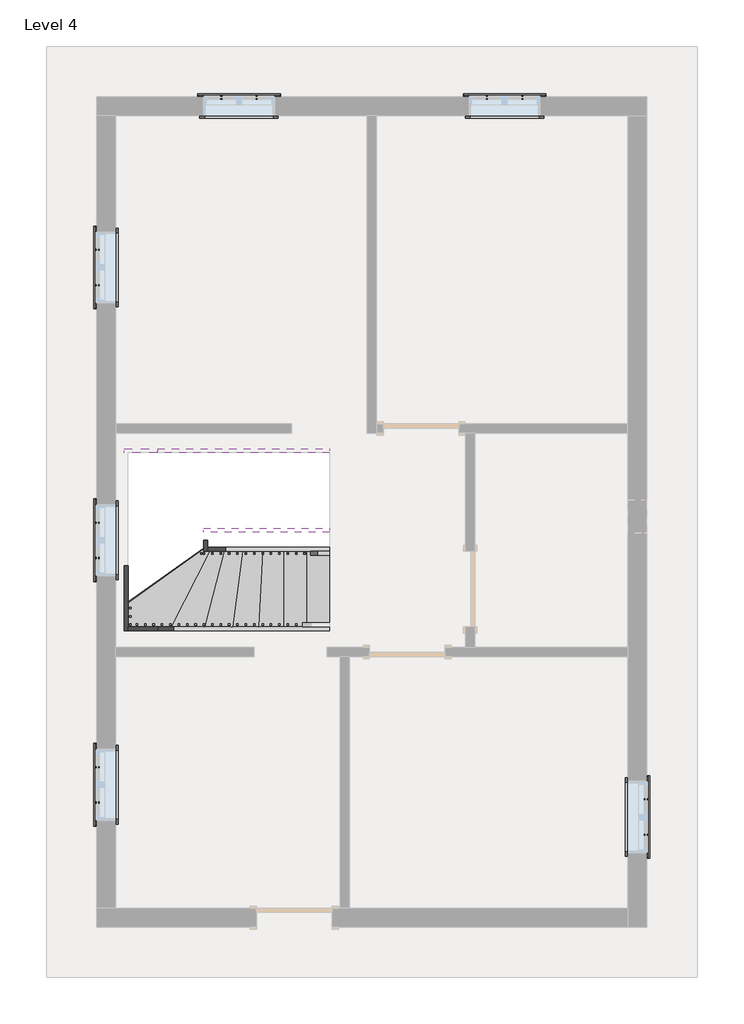
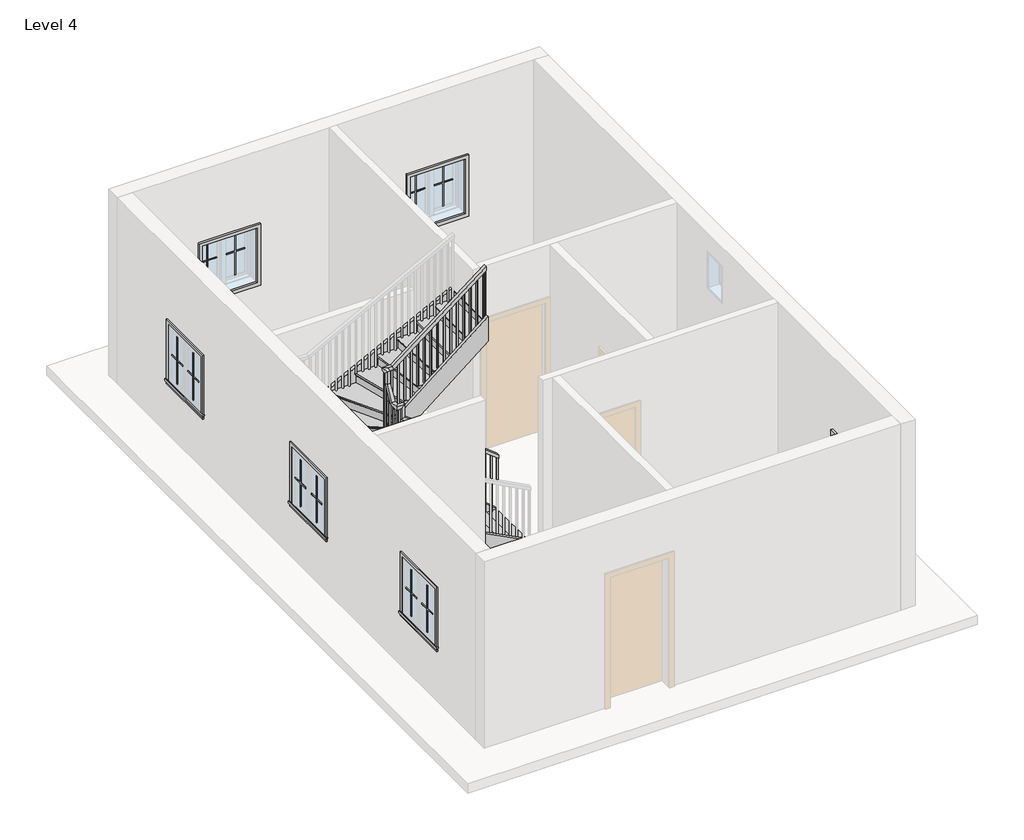
# One storey, part 2 of 2: 24 proxies, 8 members, 1 railing, 1 stair flight.
"""IFC4 building model written with IfcOpenShell, lengths in millimetres."""

from ifc_helpers import new_model, si_unit, frame, origin, place, context, project, spatial, polyline, outline, extrude, faceted_brep, transform, mapped, element, save
from components import muntin_pattern_2x2_muntin_pattern_2x2_b3fe6957, muntin_pattern_2x2_muntin_pattern_2x2_3e0ecaf2, trim_window_exterior_flat_with_sill_41619996, trim_window_interior_flat_picture_frame_51c85655, stair_flight_c61886c8

model = new_model("IFC4")

# Units and contexts
model_context = context("Model", 3, world=origin())
ifc_project = project(units=[si_unit("LENGTHUNIT", "METRE", prefix="MILLI")], contexts=[model_context])

# Site, building, storey
site = spatial("IfcSite", under=ifc_project)
building = spatial("IfcBuilding", under=site)
storey = spatial("IfcBuildingStorey", under=building, Name="Level 4", Elevation=6400.8)

# Proxies
placement = place(None, origin())
muntin_pattern_2x2_muntin_pattern_2x2_shape = muntin_pattern_2x2_muntin_pattern_2x2_b3fe6957(model_context)
element("IfcBuildingElementProxy", 1, Name="Muntin Pattern_2x2 : Muntin Pattern_2x2", ObjectType="Muntin Pattern_2x2 : Muntin Pattern_2x2", at=placement, inside=storey, context=model_context, shape_type="MappedRepresentation", body=[
    mapped(muntin_pattern_2x2_muntin_pattern_2x2_shape, transform((-3096.8324167, 5150.2179147, 7385.05), x_axis=(1.0, 0.0, 0.0), y_axis=(0.0, 1.0, 0.0), z_axis=(0.0, 0.0, 1.0))),
])
element("IfcBuildingElementProxy", 2, Name="Muntin Pattern_2x2 : Muntin Pattern_2x2", ObjectType="Muntin Pattern_2x2 : Muntin Pattern_2x2", at=placement, inside=storey, context=model_context, shape_type="MappedRepresentation", body=[
    mapped(muntin_pattern_2x2_muntin_pattern_2x2_shape, transform((122.6175833, 5150.2179147, 7385.05), x_axis=(1.0, 0.0, 0.0), y_axis=(0.0, 1.0, 0.0), z_axis=(0.0, 0.0, 1.0))),
])
element("IfcBuildingElementProxy", 3, Name="Muntin Pattern_2x2 : Muntin Pattern_2x2", ObjectType="Muntin Pattern_2x2 : Muntin Pattern_2x2", at=placement, inside=storey, context=model_context, shape_type="MappedRepresentation", body=[
    mapped(muntin_pattern_2x2_muntin_pattern_2x2_shape, transform((2051.4300833, -3350.8445853, 7385.05), x_axis=(0.0, -1.0, 0.0), y_axis=(1.0, 0.0, 0.0), z_axis=(0.0, 0.0, 1.0))),
])
element("IfcBuildingElementProxy", 4, Name="Muntin Pattern_2x2 : Muntin Pattern_2x2", ObjectType="Muntin Pattern_2x2 : Muntin Pattern_2x2", at=placement, inside=storey, context=model_context, shape_type="MappedRepresentation", body=[
    mapped(muntin_pattern_2x2_muntin_pattern_2x2_shape, transform((-4597.0199167, -426.6695853, 7385.05), x_axis=(0.0, 1.0, 0.0), y_axis=(-1.0, 0.0, 0.0), z_axis=(0.0, 0.0, 1.0))),
])
element("IfcBuildingElementProxy", 5, Name="Muntin Pattern_2x2 : Muntin Pattern_2x2", ObjectType="Muntin Pattern_2x2 : Muntin Pattern_2x2", at=placement, inside=storey, context=model_context, shape_type="MappedRepresentation", body=[
    mapped(muntin_pattern_2x2_muntin_pattern_2x2_shape, transform((-4597.0199167, -3388.9445853, 7385.05), x_axis=(0.0, 1.0, 0.0), y_axis=(-1.0, 0.0, 0.0), z_axis=(0.0, 0.0, 1.0))),
])
element("IfcBuildingElementProxy", 6, Name="Muntin Pattern_2x2 : Muntin Pattern_2x2", ObjectType="Muntin Pattern_2x2 : Muntin Pattern_2x2", at=placement, inside=storey, context=model_context, shape_type="MappedRepresentation", body=[
    mapped(muntin_pattern_2x2_muntin_pattern_2x2_shape, transform((-4597.0199167, 2878.5054147, 7385.05), x_axis=(0.0, 1.0, 0.0), y_axis=(-1.0, 0.0, 0.0), z_axis=(0.0, 0.0, 1.0))),
])
muntin_pattern_2x2_muntin_pattern_2x2_2_shape = muntin_pattern_2x2_muntin_pattern_2x2_3e0ecaf2(model_context)
element("IfcBuildingElementProxy", 7, Name="Muntin Pattern_2x2 : Muntin Pattern_2x2", ObjectType="Muntin Pattern_2x2 : Muntin Pattern_2x2", at=placement, inside=storey, context=model_context, shape_type="MappedRepresentation", body=[
    mapped(muntin_pattern_2x2_muntin_pattern_2x2_2_shape, transform((-2668.2074167, 5150.2179147, 7385.05), x_axis=(-1.0, 0.0, 0.0), y_axis=(0.0, -1.0, 0.0), z_axis=(0.0, 0.0, 1.0))),
])
element("IfcBuildingElementProxy", 8, Name="Muntin Pattern_2x2 : Muntin Pattern_2x2", ObjectType="Muntin Pattern_2x2 : Muntin Pattern_2x2", at=placement, inside=storey, context=model_context, shape_type="MappedRepresentation", body=[
    mapped(muntin_pattern_2x2_muntin_pattern_2x2_2_shape, transform((551.2425833, 5150.2179147, 7385.05), x_axis=(-1.0, 0.0, 0.0), y_axis=(0.0, -1.0, 0.0), z_axis=(0.0, 0.0, 1.0))),
])
element("IfcBuildingElementProxy", 9, Name="Muntin Pattern_2x2 : Muntin Pattern_2x2", ObjectType="Muntin Pattern_2x2 : Muntin Pattern_2x2", at=placement, inside=storey, context=model_context, shape_type="MappedRepresentation", body=[
    mapped(muntin_pattern_2x2_muntin_pattern_2x2_2_shape, transform((2051.4300833, -3779.4695853, 7385.05), x_axis=(0.0, 1.0, 0.0), y_axis=(-1.0, 0.0, 0.0), z_axis=(0.0, 0.0, 1.0))),
])
element("IfcBuildingElementProxy", 10, Name="Muntin Pattern_2x2 : Muntin Pattern_2x2", ObjectType="Muntin Pattern_2x2 : Muntin Pattern_2x2", at=placement, inside=storey, context=model_context, shape_type="MappedRepresentation", body=[
    mapped(muntin_pattern_2x2_muntin_pattern_2x2_2_shape, transform((-4597.0199167, 1.9554147, 7385.05), x_axis=(0.0, -1.0, 0.0), y_axis=(1.0, 0.0, 0.0), z_axis=(0.0, 0.0, 1.0))),
])
element("IfcBuildingElementProxy", 11, Name="Muntin Pattern_2x2 : Muntin Pattern_2x2", ObjectType="Muntin Pattern_2x2 : Muntin Pattern_2x2", at=placement, inside=storey, context=model_context, shape_type="MappedRepresentation", body=[
    mapped(muntin_pattern_2x2_muntin_pattern_2x2_2_shape, transform((-4597.0199167, -2960.3195853, 7385.05), x_axis=(0.0, -1.0, 0.0), y_axis=(1.0, 0.0, 0.0), z_axis=(0.0, 0.0, 1.0))),
])
element("IfcBuildingElementProxy", 12, Name="Muntin Pattern_2x2 : Muntin Pattern_2x2", ObjectType="Muntin Pattern_2x2 : Muntin Pattern_2x2", at=placement, inside=storey, context=model_context, shape_type="MappedRepresentation", body=[
    mapped(muntin_pattern_2x2_muntin_pattern_2x2_2_shape, transform((-4597.0199167, 3307.1304147, 7385.05), x_axis=(0.0, -1.0, 0.0), y_axis=(1.0, 0.0, 0.0), z_axis=(0.0, 0.0, 1.0))),
])
trim_window_exterior_flat_with_sill_shape = trim_window_exterior_flat_with_sill_41619996(model_context)
element("IfcBuildingElementProxy", 13, Name="Trim-Window-Exterior-Flat : with Sill", ObjectType="Trim-Window-Exterior-Flat : with Sill", at=placement, inside=storey, context=model_context, shape_type="MappedRepresentation", body=[
    mapped(trim_window_exterior_flat_with_sill_shape, transform((-2882.5199167, 5159.7429147, 8229.6), x_axis=(-1.0, 0.0, 0.0), y_axis=(0.0, 0.0, 1.0), z_axis=(0.0, 1.0, 0.0))),
])
element("IfcBuildingElementProxy", 14, Name="Trim-Window-Exterior-Flat : with Sill", ObjectType="Trim-Window-Exterior-Flat : with Sill", at=placement, inside=storey, context=model_context, shape_type="MappedRepresentation", body=[
    mapped(trim_window_exterior_flat_with_sill_shape, transform((336.9300833, 5159.7429147, 8229.6), x_axis=(-1.0, 0.0, 0.0), y_axis=(0.0, 0.0, 1.0), z_axis=(0.0, 1.0, 0.0))),
])
element("IfcBuildingElementProxy", 15, Name="Trim-Window-Exterior-Flat : with Sill", ObjectType="Trim-Window-Exterior-Flat : with Sill", at=placement, inside=storey, context=model_context, shape_type="MappedRepresentation", body=[
    mapped(trim_window_exterior_flat_with_sill_shape, transform((2060.9550833, -3565.1570853, 8229.6), x_axis=(0.0, 1.0, 0.0), y_axis=(0.0, 0.0, 1.0), z_axis=(1.0, 0.0, 0.0))),
])
element("IfcBuildingElementProxy", 16, Name="Trim-Window-Exterior-Flat : with Sill", ObjectType="Trim-Window-Exterior-Flat : with Sill", at=placement, inside=storey, context=model_context, shape_type="MappedRepresentation", body=[
    mapped(trim_window_exterior_flat_with_sill_shape, transform((-4606.5449167, -212.3570853, 8229.6), x_axis=(0.0, -1.0, 0.0), y_axis=(0.0, 0.0, 1.0), z_axis=(-1.0, 0.0, 0.0))),
])
element("IfcBuildingElementProxy", 17, Name="Trim-Window-Exterior-Flat : with Sill", ObjectType="Trim-Window-Exterior-Flat : with Sill", at=placement, inside=storey, context=model_context, shape_type="MappedRepresentation", body=[
    mapped(trim_window_exterior_flat_with_sill_shape, transform((-4606.5449167, -3174.6320853, 8229.6), x_axis=(0.0, -1.0, 0.0), y_axis=(0.0, 0.0, 1.0), z_axis=(-1.0, 0.0, 0.0))),
])
element("IfcBuildingElementProxy", 18, Name="Trim-Window-Exterior-Flat : with Sill", ObjectType="Trim-Window-Exterior-Flat : with Sill", at=placement, inside=storey, context=model_context, shape_type="MappedRepresentation", body=[
    mapped(trim_window_exterior_flat_with_sill_shape, transform((-4606.5449167, 3092.8179147, 8229.6), x_axis=(0.0, -1.0, 0.0), y_axis=(0.0, 0.0, 1.0), z_axis=(-1.0, 0.0, 0.0))),
])
trim_window_interior_flat_picture_frame_shape = trim_window_interior_flat_picture_frame_51c85655(model_context)
element("IfcBuildingElementProxy", 19, Name="Trim-Window-Interior-Flat : Picture Frame", ObjectType="Trim-Window-Interior-Flat : Picture Frame", at=placement, inside=storey, context=model_context, shape_type="MappedRepresentation", body=[
    mapped(trim_window_interior_flat_picture_frame_shape, transform((-2882.5199167, 4931.1429147, 8229.6), x_axis=(1.0, 0.0, 0.0), y_axis=(0.0, 0.0, 1.0), z_axis=(0.0, -1.0, 0.0))),
])
element("IfcBuildingElementProxy", 20, Name="Trim-Window-Interior-Flat : Picture Frame", ObjectType="Trim-Window-Interior-Flat : Picture Frame", at=placement, inside=storey, context=model_context, shape_type="MappedRepresentation", body=[
    mapped(trim_window_interior_flat_picture_frame_shape, transform((336.9300833, 4931.1429147, 8229.6), x_axis=(1.0, 0.0, 0.0), y_axis=(0.0, 0.0, 1.0), z_axis=(0.0, -1.0, 0.0))),
])
element("IfcBuildingElementProxy", 21, Name="Trim-Window-Interior-Flat : Picture Frame", ObjectType="Trim-Window-Interior-Flat : Picture Frame", at=placement, inside=storey, context=model_context, shape_type="MappedRepresentation", body=[
    mapped(trim_window_interior_flat_picture_frame_shape, transform((1832.3550833, -3565.1570853, 8229.6), x_axis=(0.0, -1.0, 0.0), y_axis=(0.0, 0.0, 1.0), z_axis=(-1.0, 0.0, 0.0))),
])
element("IfcBuildingElementProxy", 22, Name="Trim-Window-Interior-Flat : Picture Frame", ObjectType="Trim-Window-Interior-Flat : Picture Frame", at=placement, inside=storey, context=model_context, shape_type="MappedRepresentation", body=[
    mapped(trim_window_interior_flat_picture_frame_shape, transform((-4377.9449167, -212.3570853, 8229.6), x_axis=(0.0, 1.0, 0.0), y_axis=(0.0, 0.0, 1.0), z_axis=(1.0, 0.0, 0.0))),
])
element("IfcBuildingElementProxy", 23, Name="Trim-Window-Interior-Flat : Picture Frame", ObjectType="Trim-Window-Interior-Flat : Picture Frame", at=placement, inside=storey, context=model_context, shape_type="MappedRepresentation", body=[
    mapped(trim_window_interior_flat_picture_frame_shape, transform((-4377.9449167, -3174.6320853, 8229.6), x_axis=(0.0, 1.0, 0.0), y_axis=(0.0, 0.0, 1.0), z_axis=(1.0, 0.0, 0.0))),
])
element("IfcBuildingElementProxy", 24, Name="Trim-Window-Interior-Flat : Picture Frame", ObjectType="Trim-Window-Interior-Flat : Picture Frame", at=placement, inside=storey, context=model_context, shape_type="MappedRepresentation", body=[
    mapped(trim_window_interior_flat_picture_frame_shape, transform((-4377.9449167, 3092.8179147, 8229.6), x_axis=(0.0, 1.0, 0.0), y_axis=(0.0, 0.0, 1.0), z_axis=(1.0, 0.0, 0.0))),
])

# Members
element("IfcMember", 25, ObjectType="Stringer - 2\" Width", at=placement, inside=storey, context=model_context, shape_type="SweptSolid", body=[
    extrude(outline(polyline([(6400.8, -1783.4132248), (6630.439954, -1783.4132248), (7706.1956453, -3870.8304165), (7363.300629, -3870.8304165), (6400.8, -2003.1755424), (6400.8, -1783.4132248)])), frame((0.0, -1310.9070853, 0.0), z_axis=(0.0, 1.0, 0.0), x_axis=(0.0, 0.0, 1.0)), (0.0, 0.0, 1.0), 50.8),
])
element("IfcMember", 26, ObjectType="Stringer - 2\" Width", at=placement, inside=storey, context=model_context, shape_type="SweptSolid", body=[
    extrude(outline(polyline([(-3870.8304165, -1260.1070853), (-3870.8304165, -1310.9070853), (-4225.5449167, -1310.9070853), (-4225.5449167, -1260.1070853), (-3870.8304165, -1260.1070853)])), frame((0.0, 0.0, 7363.300629), z_axis=(0.0, 0.0, 1.0), x_axis=(1.0, 0.0, 0.0)), (0.0, 0.0, 1.0), 342.8950162),
])
element("IfcMember", 27, ObjectType="Stringer - 2\" Width", at=placement, inside=storey, context=model_context, shape_type="SweptSolid", body=[
    extrude(outline(polyline([(-1310.9070853, 7401.3956453), (-1310.9070853, 7689.8952212), (811.1127974, 8370.7972697), (848.0929147, 8370.7972697), (848.0929147, 8039.7682298), (-1141.3846024, 7401.3956453), (-1310.9070853, 7401.3956453)])), frame((-4276.3449167, 0.0, 0.0), z_axis=(1.0, 0.0, 0.0), x_axis=(0.0, 1.0, 0.0)), (0.0, 0.0, 1.0), 50.8),
])
element("IfcMember", 28, ObjectType="Stringer - 2\" Width", at=placement, inside=storey, context=model_context, shape_type="SweptSolid", body=[
    extrude(outline(polyline([(-4276.3449167, 848.0929147), (-4276.3449167, 898.8929147), (-3870.8304165, 898.8929147), (-3870.8304165, 848.0929147), (-4276.3449167, 848.0929147)])), frame((0.0, 0.0, 8050.6904473), z_axis=(0.0, 0.0, 1.0), x_axis=(1.0, 0.0, 0.0)), (0.0, 0.0, 1.0), 320.1068224),
])
element("IfcMember", 29, ObjectType="Stringer - 2\" Width", at=placement, inside=storey, context=model_context, shape_type="SweptSolid", body=[
    extrude(outline(polyline([(8370.7972697, -3870.8304165), (8050.6904473, -3870.8304165), (9126.4461385, -1783.4132248), (9446.5529609, -1783.4132248), (8370.7972697, -3870.8304165)])), frame((0.0, 848.0929147, 0.0), z_axis=(0.0, 1.0, 0.0), x_axis=(0.0, 0.0, 1.0)), (0.0, 0.0, 1.0), 50.8),
])
element("IfcMember", 30, ObjectType="Stringer - 2\" Width", at=placement, inside=storey, context=model_context, shape_type="SweptSolid", body=[
    extrude(outline(polyline([(6400.8, -1783.4132248), (6576.9764461, -1783.4132248), (7781.218648, -3260.3449167), (7387.9410923, -3260.3449167), (6400.8, -2049.6748694), (6400.8, -1783.4132248)])), frame((0.0, -345.7070853, 0.0), z_axis=(0.0, 1.0, 0.0), x_axis=(0.0, 0.0, 1.0)), (0.0, 0.0, 1.0), 50.8),
])
element("IfcMember", 31, ObjectType="Stringer - 2\" Width", at=placement, inside=storey, context=model_context, shape_type="SweptSolid", body=[
    extrude(outline(polyline([(-345.7070853, 7429.3617647), (-345.7070853, 7974.0682978), (-139.0699679, 8326.9409689), (-117.1070853, 8326.9409689), (-117.1070853, 7761.265107), (-311.464868, 7429.3617647), (-345.7070853, 7429.3617647)])), frame((-3311.1449167, 0.0, 0.0), z_axis=(1.0, 0.0, 0.0), x_axis=(0.0, 1.0, 0.0)), (0.0, 0.0, 1.0), 50.8),
])
element("IfcMember", 32, ObjectType="Stringer - 2\" Width", at=placement, inside=storey, context=model_context, shape_type="SweptSolid", body=[
    extrude(outline(polyline([(8326.9409689, -3311.1449167), (7933.6634131, -3311.1449167), (9179.3262875, -1783.4132248), (9572.6038432, -1783.4132248), (8326.9409689, -3311.1449167)])), frame((0.0, -117.1070853, 0.0), z_axis=(0.0, 1.0, 0.0), x_axis=(0.0, 0.0, 1.0)), (0.0, 0.0, 1.0), 50.8),
])

# Railing
element("IfcRailing", 33, ObjectType="Handrail - Rectangular", at=placement, inside=storey, context=model_context, shape_type="SolidModel", body=[
    faceted_brep([(-1783.4132248, -396.5070853, 7484.5333333), (-1783.4132248, -396.5070853, 7420.2000346), (-1783.4132248, -345.7070853, 7420.2000346), (-1783.4132248, -345.7070853, 7484.5333333), (-3234.9449167, -396.5070853, 8612.4191036), (-3285.7449167, -396.5070853, 8587.5590024), (-3285.7449167, -345.7070853, 8587.5590024), (-3234.9449167, -345.7070853, 8612.4191036), (-3234.9449167, -396.5070853, 8815.4281882), (-3285.7449167, -396.5070853, 8764.6281882), (-3285.7449167, -345.7070853, 8764.6281882), (-3234.9449167, -345.7070853, 8815.4281882), (-3361.9449167, -396.5070853, 8815.4281882), (-3361.9449167, -396.5070853, 8764.6281882), (-3311.1449167, -345.7070853, 8764.6281882), (-3311.1449167, -345.7070853, 8815.4281882), (-3361.9449167, -269.5070853, 8815.4281882), (-3361.9449167, -240.3857515, 8764.6281882), (-3311.1449167, -240.3857515, 8764.6281882), (-3311.1449167, -269.5070853, 8815.4281882), (-3361.9449167, -142.5070853, 9032.3051451), (-3361.9449167, -91.7070853, 9018.5256424), (-3311.1449167, -91.7070853, 9018.5256424), (-3311.1449167, -142.5070853, 9032.3051451), (-3361.9449167, -142.5070853, 9235.3142297), (-3361.9449167, -91.7070853, 9184.5142297), (-3311.1449167, -91.7070853, 9184.5142297), (-3311.1449167, -142.5070853, 9235.3142297), (-3361.9449167, -15.5070853, 9235.3142297), (-3361.9449167, -15.5070853, 9184.5142297), (-3311.1449167, -66.3070853, 9184.5142297), (-3311.1449167, -66.3070853, 9235.3142297), (-3234.9449167, -15.5070853, 9235.3142297), (-3217.5282487, -15.5070853, 9184.5142297), (-3217.5282487, -66.3070853, 9184.5142297), (-3234.9449167, -66.3070853, 9235.3142297), (-1783.4132248, -15.5070853, 10363.2), (-1783.4132248, -66.3070853, 10363.2), (-1783.4132248, -66.3070853, 10298.8667013), (-1783.4132248, -15.5070853, 10298.8667013)], [[[0, 1, 2, 3]], [[1, 0, 4, 5]], [[2, 1, 5, 6]], [[3, 2, 6, 7]], [[0, 3, 7, 4]], [[5, 4, 8, 9]], [[6, 5, 9, 10]], [[7, 6, 10, 11]], [[4, 7, 11, 8]], [[9, 8, 12, 13]], [[10, 9, 13, 14]], [[11, 10, 14, 15]], [[8, 11, 15, 12]], [[13, 12, 16, 17]], [[14, 13, 17, 18]], [[15, 14, 18, 19]], [[12, 15, 19, 16]], [[17, 16, 20, 21]], [[18, 17, 21, 22]], [[19, 18, 22, 23]], [[16, 19, 23, 20]], [[21, 20, 24, 25]], [[22, 21, 25, 26]], [[23, 22, 26, 27]], [[20, 23, 27, 24]], [[25, 24, 28, 29]], [[26, 25, 29, 30]], [[27, 26, 30, 31]], [[24, 27, 31, 28]], [[29, 28, 32, 33]], [[30, 29, 33, 34]], [[31, 30, 34, 35]], [[28, 31, 35, 32]], [[36, 37, 38, 39]], [[33, 32, 36, 39]], [[34, 33, 39, 38]], [[35, 34, 38, 37]], [[32, 35, 37, 36]]]),
    extrude(outline(polyline([(10283.6316852, -1803.0199167), (10268.8292361, -1822.0699167), (9279.4666667, -1822.0699167), (9279.4666667, -1803.0199167), (10283.6316852, -1803.0199167)])), frame((0.0, -50.4320853, 0.0), z_axis=(0.0, 1.0, 0.0), x_axis=(0.0, 0.0, 1.0)), (0.0, 0.0, 1.0), 19.05),
    extrude(outline(polyline([(10204.6852902, -1904.6199167), (10189.8828411, -1923.6699167), (9279.4666667, -1923.6699167), (9279.4666667, -1904.6199167), (10204.6852902, -1904.6199167)])), frame((0.0, -50.4320853, 0.0), z_axis=(0.0, 1.0, 0.0), x_axis=(0.0, 0.0, 1.0)), (0.0, 0.0, 1.0), 19.05),
    extrude(outline(polyline([(10125.7388952, -2006.2199167), (10110.9364462, -2025.2699167), (9279.4666667, -2025.2699167), (9279.4666667, -2006.2199167), (10125.7388952, -2006.2199167)])), frame((0.0, -50.4320853, 0.0), z_axis=(0.0, 1.0, 0.0), x_axis=(0.0, 0.0, 1.0)), (0.0, 0.0, 1.0), 19.05),
    extrude(outline(polyline([(10046.7925003, -2107.8199167), (10031.9900512, -2126.8699167), (9110.1333333, -2126.8699167), (9110.1333333, -2107.8199167), (10046.7925003, -2107.8199167)])), frame((0.0, -50.4320853, 0.0), z_axis=(0.0, 1.0, 0.0), x_axis=(0.0, 0.0, 1.0)), (0.0, 0.0, 1.0), 19.05),
    extrude(outline(polyline([(9967.8461053, -2209.4199167), (9953.0436562, -2228.4699167), (9110.1333333, -2228.4699167), (9110.1333333, -2209.4199167), (9967.8461053, -2209.4199167)])), frame((0.0, -50.4320853, 0.0), z_axis=(0.0, 1.0, 0.0), x_axis=(0.0, 0.0, 1.0)), (0.0, 0.0, 1.0), 19.05),
    extrude(outline(polyline([(9888.8997103, -2311.0199167), (9874.0972613, -2330.0699167), (9110.1333333, -2330.0699167), (9110.1333333, -2311.0199167), (9888.8997103, -2311.0199167)])), frame((0.0, -50.4320853, 0.0), z_axis=(0.0, 1.0, 0.0), x_axis=(0.0, 0.0, 1.0)), (0.0, 0.0, 1.0), 19.05),
    extrude(outline(polyline([(9809.9533154, -2412.6199167), (9795.1508663, -2431.6699167), (8940.8, -2431.6699167), (8940.8, -2412.6199167), (9809.9533154, -2412.6199167)])), frame((0.0, -50.4320853, 0.0), z_axis=(0.0, 1.0, 0.0), x_axis=(0.0, 0.0, 1.0)), (0.0, 0.0, 1.0), 19.05),
    extrude(outline(polyline([(9731.0069204, -2514.2199167), (9716.2044713, -2533.2699167), (8940.8, -2533.2699167), (8940.8, -2514.2199167), (9731.0069204, -2514.2199167)])), frame((0.0, -50.4320853, 0.0), z_axis=(0.0, 1.0, 0.0), x_axis=(0.0, 0.0, 1.0)), (0.0, 0.0, 1.0), 19.05),
    extrude(outline(polyline([(9652.0605254, -2615.8199167), (9637.2580764, -2634.8699167), (8771.4666667, -2634.8699167), (8771.4666667, -2615.8199167), (9652.0605254, -2615.8199167)])), frame((0.0, -50.4320853, 0.0), z_axis=(0.0, 1.0, 0.0), x_axis=(0.0, 0.0, 1.0)), (0.0, 0.0, 1.0), 19.05),
    extrude(outline(polyline([(9573.1141304, -2717.4199167), (9558.3116814, -2736.4699167), (8771.4666667, -2736.4699167), (8771.4666667, -2717.4199167), (9573.1141304, -2717.4199167)])), frame((0.0, -50.4320853, 0.0), z_axis=(0.0, 1.0, 0.0), x_axis=(0.0, 0.0, 1.0)), (0.0, 0.0, 1.0), 19.05),
    extrude(outline(polyline([(9494.1677355, -2819.0199167), (9479.3652864, -2838.0699167), (8771.4666667, -2838.0699167), (8771.4666667, -2819.0199167), (9494.1677355, -2819.0199167)])), frame((0.0, -50.4320853, 0.0), z_axis=(0.0, 1.0, 0.0), x_axis=(0.0, 0.0, 1.0)), (0.0, 0.0, 1.0), 19.05),
    extrude(outline(polyline([(9415.2213405, -2920.6199167), (9400.4188914, -2939.6699167), (8602.1333333, -2939.6699167), (8602.1333333, -2920.6199167), (9415.2213405, -2920.6199167)])), frame((0.0, -50.4320853, 0.0), z_axis=(0.0, 1.0, 0.0), x_axis=(0.0, 0.0, 1.0)), (0.0, 0.0, 1.0), 19.05),
    extrude(outline(polyline([(9336.2749455, -3022.2199167), (9321.4724965, -3041.2699167), (8602.1333333, -3041.2699167), (8602.1333333, -3022.2199167), (9336.2749455, -3022.2199167)])), frame((0.0, -50.4320853, 0.0), z_axis=(0.0, 1.0, 0.0), x_axis=(0.0, 0.0, 1.0)), (0.0, 0.0, 1.0), 19.05),
    extrude(outline(polyline([(9257.3285506, -3123.8199167), (9242.5261015, -3142.8699167), (8432.8, -3142.8699167), (8432.8, -3123.8199167), (9257.3285506, -3123.8199167)])), frame((0.0, -50.4320853, 0.0), z_axis=(0.0, 1.0, 0.0), x_axis=(0.0, 0.0, 1.0)), (0.0, 0.0, 1.0), 19.05),
    extrude(outline(polyline([(9178.3821556, -3225.4199167), (9163.5797065, -3244.4699167), (8432.8, -3244.4699167), (8432.8, -3225.4199167), (9178.3821556, -3225.4199167)])), frame((0.0, -50.4320853, 0.0), z_axis=(0.0, 1.0, 0.0), x_axis=(0.0, 0.0, 1.0)), (0.0, 0.0, 1.0), 19.05),
    extrude(outline(polyline([(-3327.0199167, -75.8320853), (-3346.0699167, -75.8320853), (-3346.0699167, -56.7820853), (-3327.0199167, -56.7820853), (-3327.0199167, -75.8320853)])), frame((0.0, 0.0, 8094.1333333), z_axis=(0.0, 0.0, 1.0), x_axis=(1.0, 0.0, 0.0)), (0.0, 0.0, 1.0), 1090.3808964),
    extrude(outline(polyline([(-177.4320853, 8872.1336964), (-158.3820853, 8904.66524), (-158.3820853, 7924.8), (-177.4320853, 7924.8), (-177.4320853, 8872.1336964)])), frame((-3346.0699167, 0.0, 0.0), z_axis=(1.0, 0.0, 0.0), x_axis=(0.0, 1.0, 0.0)), (0.0, 0.0, 1.0), 19.05),
    extrude(outline(polyline([(-279.0320853, 8698.6321309), (-259.9820853, 8731.1636744), (-259.9820853, 7755.4666667), (-279.0320853, 7755.4666667), (-279.0320853, 8698.6321309)])), frame((-3346.0699167, 0.0, 0.0), z_axis=(1.0, 0.0, 0.0), x_axis=(0.0, 1.0, 0.0)), (0.0, 0.0, 1.0), 19.05),
    extrude(outline(polyline([(-3297.8882248, -361.5820853), (-3297.8882248, -380.6320853), (-3316.9382248, -380.6320853), (-3316.9382248, -361.5820853), (-3297.8882248, -361.5820853)])), frame((0.0, 0.0, 7586.1333333), z_axis=(0.0, 0.0, 1.0), x_axis=(1.0, 0.0, 0.0)), (0.0, 0.0, 1.0), 1178.4948549),
    extrude(outline(polyline([(8518.0483397, -3196.2882248), (8532.8507888, -3215.3382248), (7416.8, -3215.3382248), (7416.8, -3196.2882248), (8518.0483397, -3196.2882248)])), frame((0.0, -380.6320853, 0.0), z_axis=(0.0, 1.0, 0.0), x_axis=(0.0, 0.0, 1.0)), (0.0, 0.0, 1.0), 19.05),
    extrude(outline(polyline([(8439.1019447, -3094.6882248), (8453.9043938, -3113.7382248), (7416.8, -3113.7382248), (7416.8, -3094.6882248), (8439.1019447, -3094.6882248)])), frame((0.0, -380.6320853, 0.0), z_axis=(0.0, 1.0, 0.0), x_axis=(0.0, 0.0, 1.0)), (0.0, 0.0, 1.0), 19.05),
    extrude(outline(polyline([(8360.1555498, -2993.0882248), (8374.9579988, -3012.1382248), (7247.4666667, -3012.1382248), (7247.4666667, -2993.0882248), (8360.1555498, -2993.0882248)])), frame((0.0, -380.6320853, 0.0), z_axis=(0.0, 1.0, 0.0), x_axis=(0.0, 0.0, 1.0)), (0.0, 0.0, 1.0), 19.05),
    extrude(outline(polyline([(8281.2091548, -2891.4882248), (8296.0116039, -2910.5382248), (7247.4666667, -2910.5382248), (7247.4666667, -2891.4882248), (8281.2091548, -2891.4882248)])), frame((0.0, -380.6320853, 0.0), z_axis=(0.0, 1.0, 0.0), x_axis=(0.0, 0.0, 1.0)), (0.0, 0.0, 1.0), 19.05),
    extrude(outline(polyline([(8202.2627598, -2789.8882248), (8217.0652089, -2808.9382248), (7078.1333333, -2808.9382248), (7078.1333333, -2789.8882248), (8202.2627598, -2789.8882248)])), frame((0.0, -380.6320853, 0.0), z_axis=(0.0, 1.0, 0.0), x_axis=(0.0, 0.0, 1.0)), (0.0, 0.0, 1.0), 19.05),
    extrude(outline(polyline([(8123.3163649, -2688.2882248), (8138.1188139, -2707.3382248), (7078.1333333, -2707.3382248), (7078.1333333, -2688.2882248), (8123.3163649, -2688.2882248)])), frame((0.0, -380.6320853, 0.0), z_axis=(0.0, 1.0, 0.0), x_axis=(0.0, 0.0, 1.0)), (0.0, 0.0, 1.0), 19.05),
    extrude(outline(polyline([(8044.3699699, -2586.6882248), (8059.1724189, -2605.7382248), (6908.8, -2605.7382248), (6908.8, -2586.6882248), (8044.3699699, -2586.6882248)])), frame((0.0, -380.6320853, 0.0), z_axis=(0.0, 1.0, 0.0), x_axis=(0.0, 0.0, 1.0)), (0.0, 0.0, 1.0), 19.05),
    extrude(outline(polyline([(7965.4235749, -2485.0882248), (7980.226024, -2504.1382248), (6908.8, -2504.1382248), (6908.8, -2485.0882248), (7965.4235749, -2485.0882248)])), frame((0.0, -380.6320853, 0.0), z_axis=(0.0, 1.0, 0.0), x_axis=(0.0, 0.0, 1.0)), (0.0, 0.0, 1.0), 19.05),
    extrude(outline(polyline([(7886.4771799, -2383.4882248), (7901.279629, -2402.5382248), (6908.8, -2402.5382248), (6908.8, -2383.4882248), (7886.4771799, -2383.4882248)])), frame((0.0, -380.6320853, 0.0), z_axis=(0.0, 1.0, 0.0), x_axis=(0.0, 0.0, 1.0)), (0.0, 0.0, 1.0), 19.05),
    extrude(outline(polyline([(7807.530785, -2281.8882248), (7822.333234, -2300.9382248), (6739.4666667, -2300.9382248), (6739.4666667, -2281.8882248), (7807.530785, -2281.8882248)])), frame((0.0, -380.6320853, 0.0), z_axis=(0.0, 1.0, 0.0), x_axis=(0.0, 0.0, 1.0)), (0.0, 0.0, 1.0), 19.05),
    extrude(outline(polyline([(7728.58439, -2180.2882248), (7743.3868391, -2199.3382248), (6739.4666667, -2199.3382248), (6739.4666667, -2180.2882248), (7728.58439, -2180.2882248)])), frame((0.0, -380.6320853, 0.0), z_axis=(0.0, 1.0, 0.0), x_axis=(0.0, 0.0, 1.0)), (0.0, 0.0, 1.0), 19.05),
    extrude(outline(polyline([(7649.637995, -2078.6882248), (7664.4404441, -2097.7382248), (6739.4666667, -2097.7382248), (6739.4666667, -2078.6882248), (7649.637995, -2078.6882248)])), frame((0.0, -380.6320853, 0.0), z_axis=(0.0, 1.0, 0.0), x_axis=(0.0, 0.0, 1.0)), (0.0, 0.0, 1.0), 19.05),
    extrude(outline(polyline([(7570.6916001, -1977.0882248), (7585.4940491, -1996.1382248), (6570.1333333, -1996.1382248), (6570.1333333, -1977.0882248), (7570.6916001, -1977.0882248)])), frame((0.0, -380.6320853, 0.0), z_axis=(0.0, 1.0, 0.0), x_axis=(0.0, 0.0, 1.0)), (0.0, 0.0, 1.0), 19.05),
    extrude(outline(polyline([(7491.7452051, -1875.4882248), (7506.5476541, -1894.5382248), (6570.1333333, -1894.5382248), (6570.1333333, -1875.4882248), (7491.7452051, -1875.4882248)])), frame((0.0, -380.6320853, 0.0), z_axis=(0.0, 1.0, 0.0), x_axis=(0.0, 0.0, 1.0)), (0.0, 0.0, 1.0), 19.05),
    extrude(outline(polyline([(-3327.0199167, -50.4320853), (-3346.0699167, -50.4320853), (-3346.0699167, -31.3820853), (-3327.0199167, -31.3820853), (-3327.0199167, -50.4320853)])), frame((0.0, 0.0, 8263.4666667), z_axis=(0.0, 0.0, 1.0), x_axis=(1.0, 0.0, 0.0)), (0.0, 0.0, 1.0), 921.0475631),
    extrude(outline(polyline([(-3327.0199167, -361.5820853), (-3327.0199167, -380.6320853), (-3346.0699167, -380.6320853), (-3346.0699167, -361.5820853), (-3327.0199167, -361.5820853)])), frame((0.0, 0.0, 7586.1333333), z_axis=(0.0, 0.0, 1.0), x_axis=(1.0, 0.0, 0.0)), (0.0, 0.0, 1.0), 1178.4948549),
    extrude(outline(polyline([(10298.8667013, -1783.4132248), (10284.0642523, -1802.4632248), (9279.4666667, -1802.4632248), (9279.4666667, -1783.4132248), (10298.8667013, -1783.4132248)])), frame((0.0, -50.4320853, 0.0), z_axis=(0.0, 1.0, 0.0), x_axis=(0.0, 0.0, 1.0)), (0.0, 0.0, 1.0), 19.05),
    extrude(outline(polyline([(7420.2000346, -1783.4132248), (7435.0024837, -1802.4632248), (6570.1333333, -1802.4632248), (6570.1333333, -1783.4132248), (7420.2000346, -1783.4132248)])), frame((0.0, -380.6320853, 0.0), z_axis=(0.0, 1.0, 0.0), x_axis=(0.0, 0.0, 1.0)), (0.0, 0.0, 1.0), 19.05),
])

# Stair flight
stair_flight_shape = stair_flight_c61886c8(model_context)
element("IfcStairFlight", 34, ObjectType="2\" Tread 1\" Nosing 1/4\" Riser", at=placement, inside=storey, context=model_context, shape_type="MappedRepresentation", body=[
    mapped(stair_flight_shape, transform((0.0, 0.0, 0.0), x_axis=(1.0, 0.0, 0.0), y_axis=(0.0, 1.0, 0.0), z_axis=(0.0, 0.0, 1.0))),
])

save(model, "model.ifc")

# Revit data of these elements
# Type "Muntin Pattern_2x2 : Muntin Pattern_2x2"
#   Width [instance default] = 4' - 0"
#   Thickness = 0' - 0 1/2"
#   Height [instance default] = 4' - 0"
#   Distance = 0' - 0 3/4"
#   Interior Material [instance default] = none
#   Exterior Material [instance default] = none
#   Default Elevation = 0
# Type "Trim-Window-Exterior-Flat : with Sill"
#   Trim Width = 0' - 2 1/4"
#   Trim Thickness_Picture Frame = 0' - 1 1/4"
#   Trim Thickness_with Sill = 0' - 0 3/4"
#   Sill Thickness = 0' - 1 1/4"
#   Opening Width [instance default] = 2' - 0"
#   Opening Height [instance default] = 3' - 0"
#   Default Elevation = 4' - 0"
#   Sill = yes
#   Picture Frame = no
#   Trim Material [instance default] = none
# Type "Trim-Window-Interior-Flat : Picture Frame"
#   Trim Thickness_Picture Frame = 0' - 1 1/4"
#   Trim Width = 0' - 2 1/4"
#   Trim Thickness_with Sill = 0' - 0 3/4"
#   Sill Thickness = 0' - 1 1/4"
#   Opening Width [instance default] = 2' - 0"
#   Opening Height [instance default] = 3' - 0"
#   Default Elevation = 4' - 0"
#   Sill = no
#   Picture Frame = yes
#   Trim Material [instance default] = none
# Type "Handrail - Rectangular"
#   Assembly Code = "C2010400"
#   built-in parameter 1008612 = 0.0416667 (stored number, unit not read)
#   built-in parameter 1008611 = 0.0416667 (stored number, unit not read)
#   built-in parameter 1008609 = 0.333333 (stored number, unit not read)
#   built-in parameter 1008604 = 0.166667 (stored number, unit not read)
#   built-in parameter 1008603 = 0.166667 (stored number, unit not read)
#   Railing Height = 3' - 0"
#   built-in parameter 1008630 = 2
#   built-in parameter 1008610 = 2
#   built-in parameter 1008618 = Baluster - Square : 3/4"
# Elements 1, 2, 3, 4, 5, 6, 7, 8, 9, 10, 11, 12 (IfcBuildingElementProxy, "Muntin Pattern_2x2 : Muntin Pattern_2x2")
#   Width = 0' - 11 5/8"
#   Height = 2' - 6 1/2"
#   Interior Material = Wood - Stained
#   Exterior Material = Clad - White
#   Phase Created = New Construction
#   Materials on its faces: "Clad - White", "Wood - Stained"
# Elements 13, 14, 15, 16, 17, 18 (IfcBuildingElementProxy, "Trim-Window-Exterior-Flat : with Sill")
#   Opening Width = 2' - 10"
#   Opening Height = 3' - 0"
#   Trim Material = Clad - White
#   Phase Created = New Construction
#   Materials on its faces: "Clad - White"
# Elements 19, 20, 21, 22, 23, 24 (IfcBuildingElementProxy, "Trim-Window-Interior-Flat : Picture Frame")
#   Opening Width = 2' - 10"
#   Opening Height = 3' - 0"
#   Trim Material = Wood - Stained
#   Phase Created = New Construction
#   Materials on its faces: "Wood - Stained"
# Elements 25, 26, 27, 28, 29, 30, 31, 32 (IfcMember, "Stringer - 2\" Width")
#   Phase Created = New Construction
# Element 33 (IfcRailing, "Handrail - Rectangular")
#   Phase Created = New Construction
# Element 34 (IfcStairFlight, "2\" Tread 1\" Nosing 1/4\" Riser")
#   Phase Created = New Construction
# Materials
#   "Clad - White": class "Wood", colour RGB 242 242 238, transparency 0, Cost = 0
#   "Wood - Stained": class "Wood", colour RGB 224 178 126, transparency 0, Cost = 0
